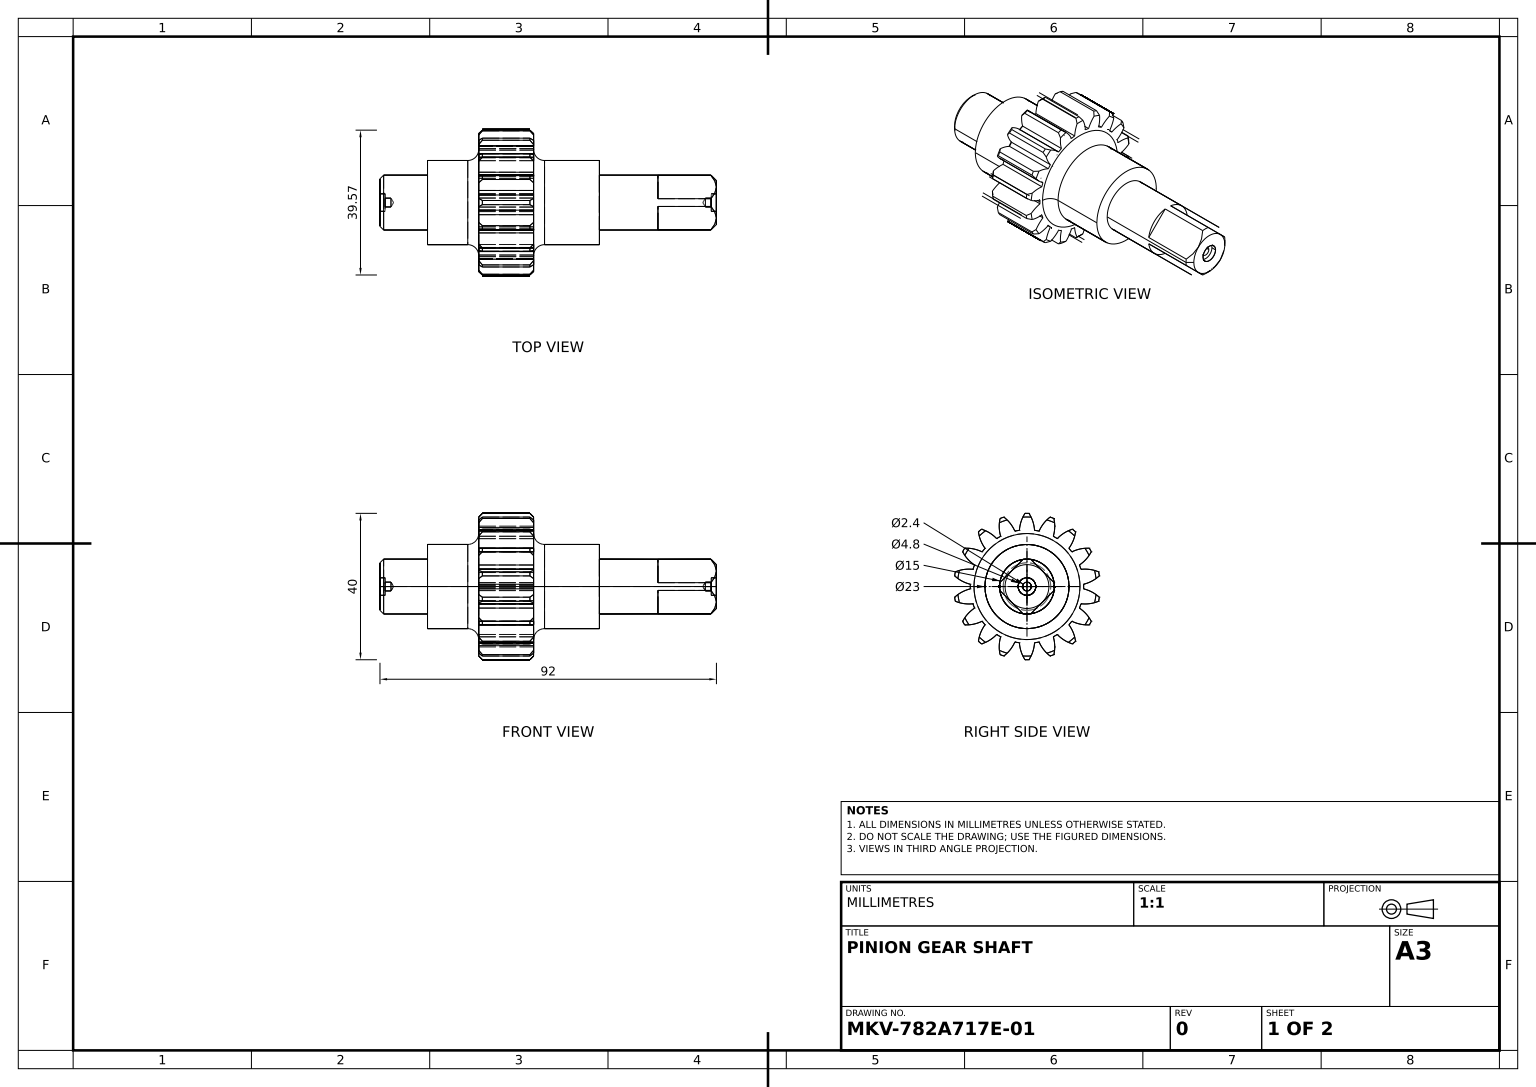
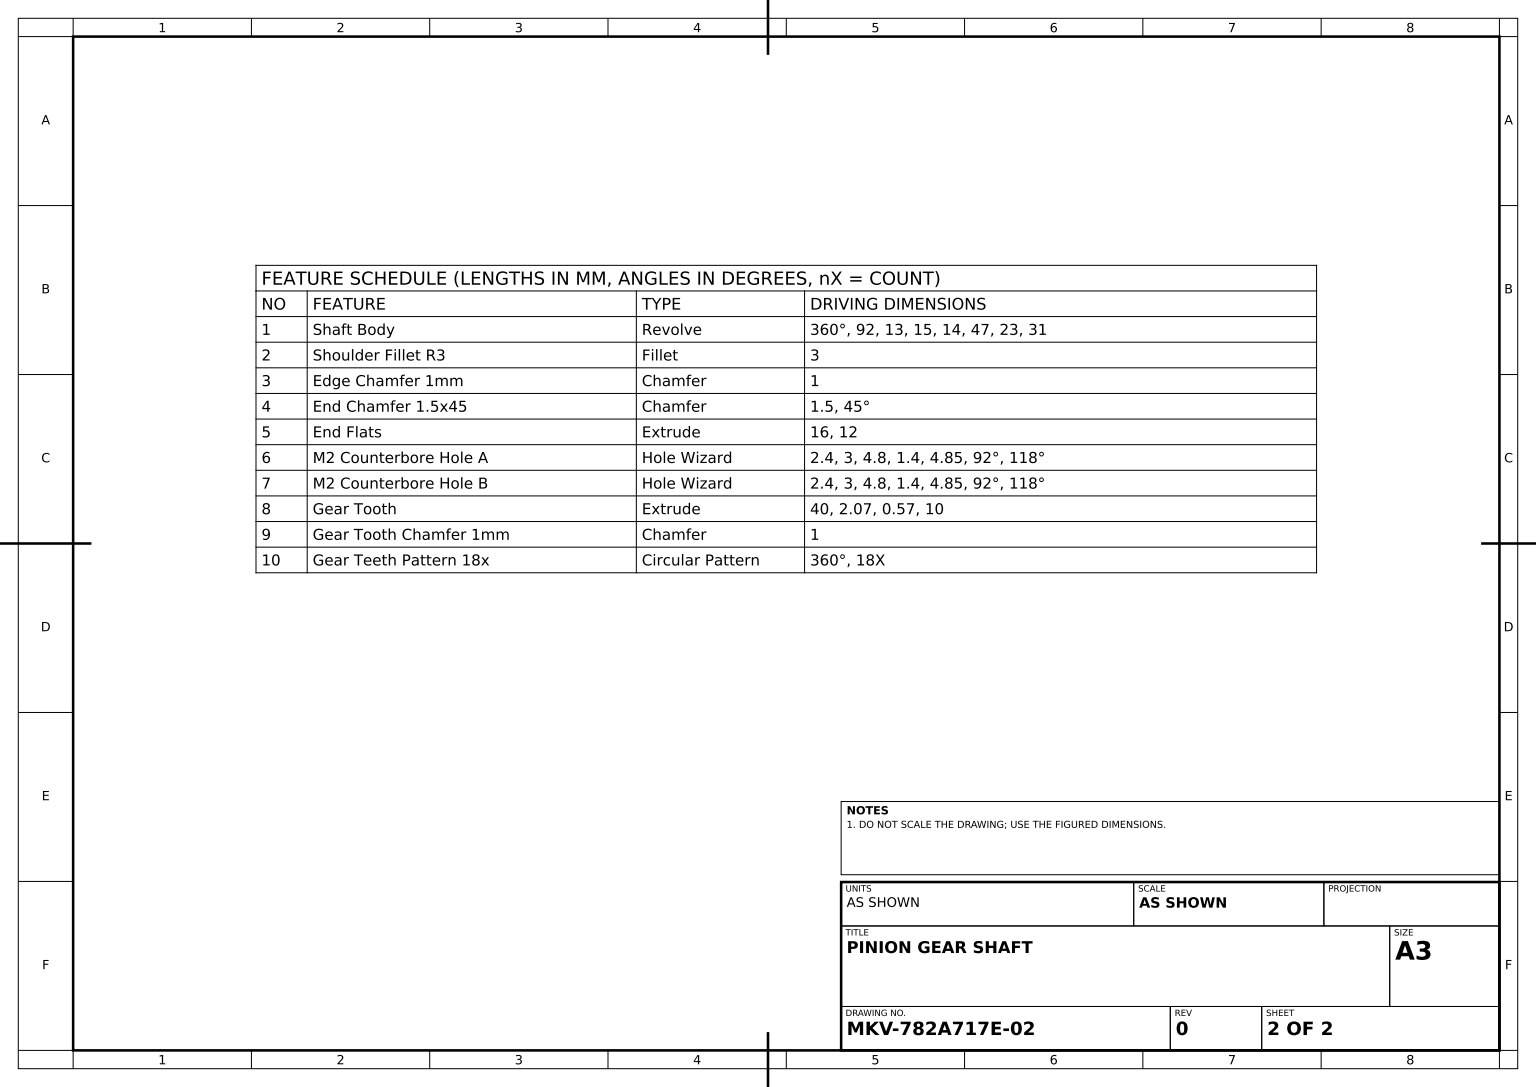
SolidWorks part; units mm, degrees
material "Plain Carbon Steel"
ref_plane "Front Plane" through (0, 0, 0) normal (0, 0, 1) x (1, 0, 0)
ref_plane "Top Plane" through (0, 0, 0) normal (0, 1, 0) x (1, 0, 0)
ref_plane "Right Plane" through (0, 0, 0) normal (1, 0, 0) x (0, 0, -1)
sketch "Shaft Profile" plane through (0, 0, 0) normal (0, 0, 1) x (1, 0, 0)
  line L0 (-34.5, 0) -> (57.5, 0) construction
  line L1 (-34.5, 0) -> (-34.5, -7.5)
  line L2 (-34.5, -7.5) -> (-21.5, -7.5)
  line L3 (-21.5, -7.5) -> (-21.5, -11.5)
  line L4 (-21.5, -11.5) -> (-7.5, -11.5)
  line L5 (-7.5, -11.5) -> (-7.5, -15.5)
  line L6 (-7.5, -15.5) -> (7.5, -15.5)
  line L7 (7.5, -15.5) -> (7.5, -11.5)
  line L8 (7.5, -11.5) -> (25.5, -11.5)
  line L9 (25.5, -11.5) -> (25.5, -7.5)
  line L10 (25.5, -7.5) -> (57.5, -7.5)
  line L11 (57.5, -7.5) -> (57.5, 0)
  line L12 (-34.5, 0) -> (57.5, 0)
  point P17 (0, -15.5)
  dimension "D1" = 92
  dimension "D2" = 15
  dimension "D3" = 23
  dimension "D4" = 31
  dimension "D5" = 13
  dimension "D6" = 15
  dimension "D7" = 14
  dimension "D8" = 47
revolve "Shaft Body" add sketch "Shaft Profile" angle 360 about L0
fillet "Shoulder Fillet R3" radius 3 2 edges at (-7.5, 0, 11.5) (7.5, 0, 11.5)
chamfer "Edge Chamfer 1mm" distance 1 1 edges at (-34.5, 0, 7.5)
chamfer "End Chamfer 1.5x45" distance 1.5 angle 45 1 edges at (57.5, 0, 7.5)
sketch "End Flats Profile" plane through (57.5, 0, 0) normal (1, 0, 0) x (0, 0, -1)
  line L0 (0, 0) -> (8.4853, 0) construction
  line L1 (0, -8.4853) -> (8.4853, 0)
  line L2 (8.4853, 0) -> (0, 8.4853)
  line L3 (0, 8.4853) -> (-8.4853, 0)
  line L4 (-8.4853, 0) -> (0, -8.4853)
  circle A0 centre (0, 0) radius 6 construction
  circle A1 centre (0, 0) radius 7.5 construction
  circle A2 centre (0, 0) radius 7.5
  dimension "D1" = 12
extrude "End Flats" cut sketch "End Flats Profile" against normal blind 16 contours L3 A2 | L4 A2 | L1 A2 | L2 A2
hole_wizard "M2 Counterbore Hole A" positions "Sketch4" profile "Sketch5" counterbore size "M2" standard "KS"
sketch "Sketch4" plane through (57.5, 0, 0) normal (1, 0, 0) x (0, 0, -1)
  point P0 (0, 0)
sketch "Sketch5" plane through (57.5, 0, 0) normal (0, 1, 0) x (0, 0, -1)
  line L0 (0, 0) -> (0, 3.721)
  line L1 (0, 3.721) -> (1.2, 3)
  line L2 (1.2, 3) -> (1.2, 1.4)
  line L3 (1.2, 1.4) -> (2.4, 1.4)
  line L5 (2.4, 1.4) -> (2.4, 0.0241)
  line L6 (2.4, 0.0241) -> (2.425, 0)
  line L7 (2.425, 0) -> (0, 0)
  line L8 (-2.4, 0.0241) -> (-2.425, 0) construction
  line L10 (0, 3.721) -> (-1.2, 3) construction
  line L11 (0, -6.35) -> (0, 107.95) construction
  dimension "Hole Dia." = 2.4
  dimension "Hole Depth" = 3
  dimension "C'Bore Dia." = 4.8
  dimension "C'Bore Depth" = 1.4
  dimension "Near C'Sink Dia." = 4.85
  dimension "Near C'Sink Angle" = 92
  dimension "Drill Angle" = 118
hole_wizard "M2 Counterbore Hole B" positions "Sketch6" profile "Sketch7" counterbore size "M2" standard "KS"
sketch "Sketch6" plane through (-34.5, 0, 0) normal (-1, 0, 0) x (0, 0, 1)
  point P0 (0, 0)
sketch "Sketch7" plane through (-34.5, 0, 0) normal (0, 1, 0) x (0, 0, 1)
  line L0 (0, 0) -> (0, 3.721)
  line L1 (0, 3.721) -> (1.2, 3)
  line L2 (1.2, 3) -> (1.2, 1.4)
  line L3 (1.2, 1.4) -> (2.4, 1.4)
  line L5 (2.4, 1.4) -> (2.4, 0.0241)
  line L6 (2.4, 0.0241) -> (2.425, 0)
  line L7 (2.425, 0) -> (0, 0)
  line L8 (-2.4, 0.0241) -> (-2.425, 0) construction
  line L10 (0, 3.721) -> (-1.2, 3) construction
  line L11 (0, -6.35) -> (0, 107.95) construction
  dimension "Hole Dia." = 2.4
  dimension "Hole Depth" = 3
  dimension "C'Bore Dia." = 4.8
  dimension "C'Bore Depth" = 1.4
  dimension "Near C'Sink Dia." = 4.85
  dimension "Near C'Sink Angle" = 92
  dimension "Drill Angle" = 118
sketch "Gear Tooth Profile" plane through (7.5, 0, 0) normal (1, 0, 0) x (0, 0, -1)
  line L0 (0, 0) -> (0, 20) construction
  arc A0 (0.57, 19.9919) -> (-0.57, 19.9919) centre (0, 0) ccw
  circle A1 centre (0, 0) radius 15.5 construction
  arc A2 (2.07, 15.3612) -> (-2.07, 15.3612) centre (0, 0) ccw
  arc A3 (-2.07, 15.3612) -> (-0.57, 19.9919) centre (7.9073, 14.6876) cw
  arc A4 (2.07, 15.3612) -> (0.57, 19.9919) centre (-7.9073, 14.6876) ccw
  dimension "D1" = 40
  dimension "D4" = 10
  dimension "D2" = 2.07
  dimension "D3" = 0.57
extrude "Gear Tooth" add sketch "Gear Tooth Profile" against normal up to surface (15 mm away) up to face at (-7.5, 0, 14.5)
chamfer "Gear Tooth Chamfer 1mm" distance 1 2 edges at (-7.5, 20, 0) (7.5, 20, 0)
pattern_circular "Gear Teeth Pattern 18x" count 18 over 360 about axis through (0, 0, 0) along (1, 0, 0) of "Gear Tooth Chamfer 1mm", "Gear Tooth"
